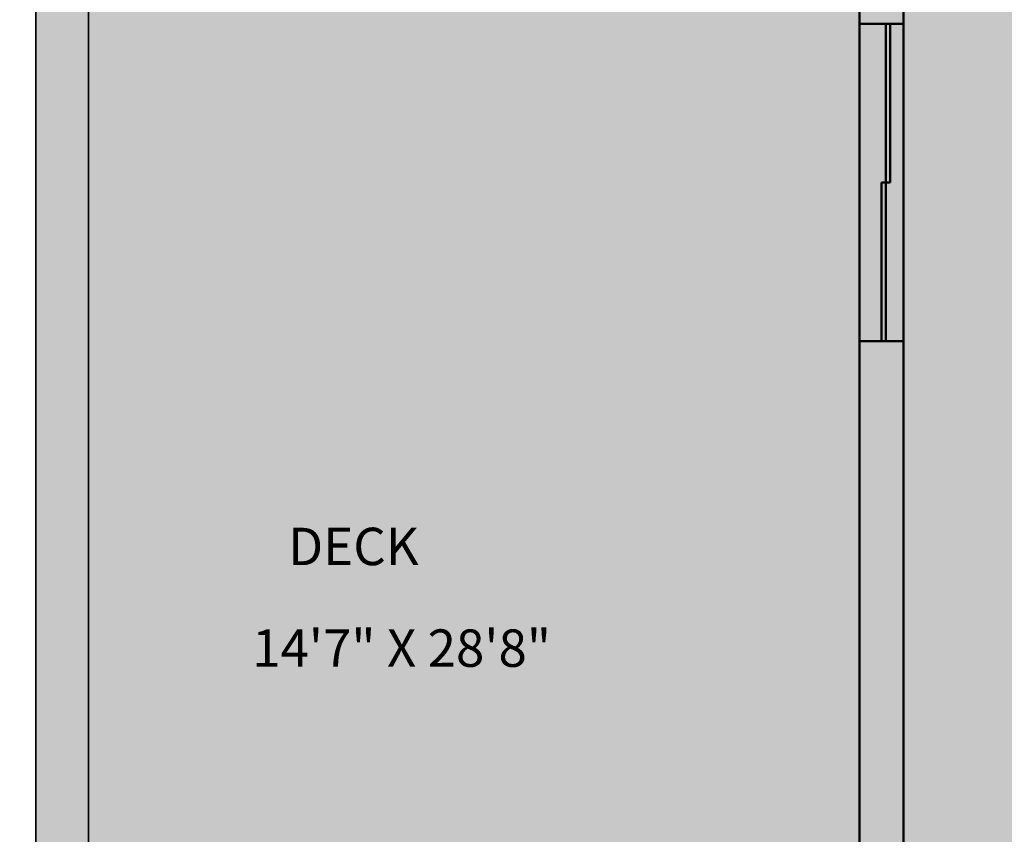
# Model space of a CAD drawing. Units: inches. Extents: x 925 to 2834, y 111 to 1355.
# Tile 14 of 25: x 1069 to 1293, y 882 to 1067. Entities that reach past the tile are written whole.
import ezdxf

# ---------------------------------------------------------------- set-up
doc = ezdxf.new("R2010")
doc.units = ezdxf.units.IN
doc.header["$MEASUREMENT"] = 0
for name, color, linetype, lineweight in [('A-ANNO-DIMS', 2, 'Continuous', 18), ('A-ANNO-TTLB', 7, 'Continuous', 35), ('A-AREA-IDEN', 7, 'Continuous', 18), ('A-FLOR-PATT', 252, 'Continuous', 13), ('A-WALL', 7, 'Continuous', 50), ('A-WALL-PATT', 8, 'Continuous', 13)]:
    doc.layers.add(name, color=color, linetype=linetype, lineweight=lineweight)
doc.styles.get("Standard").update_dxf_attribs({"font": 'arial.ttf'})
doc.dimstyles.get("Standard").update_dxf_attribs({"dimtxt": 6, "dimasz": 3, "dimexe": 0.18, "dimexo": 0.0625, "dimgap": 0.09, "dimtad": 0, "dimtih": 1, "dimtoh": 1, "dimdec": 1, "dimzin": 0, "dimdsep": 46, "dimlunit": 3, "dimtxsty": 'Standard', "dimblk": 'ARCHTICK', "dimcen": 0.09, "dimadec": 0, "dimazin": 0, "dimtfac": 1, "dimtdec": 1, "dimtofl": 0, "dimtmove": 0, "dimatfit": 3, "dimfxl": 1, "dimtolj": 1, "dimtzin": 0, "dimarcsym": 0})

# ---------------------------------------------------------------- blocks, each defined once
blk = doc.blocks.new('_ArchTick')
at = {"color": 0, "linetype": 'ByBlock', "const_width": 0.15}
blk.add_lwpolyline([(-0.5, -0.5), (0.5, 0.5)], dxfattribs=at)
blk = doc.blocks.new('*D36')
at = {"layer": 'A-ANNO-DIMS', "color": 0, "lineweight": -2, "transparency": 16777216}
for p, q in [((1084.65, 1081.59), (934.81, 1081.59)), ((934.99, 1081.59), (934.99, 907.74)), ((934.99, 727.59), (934.99, 901.43)), ((1084.65, 727.59), (934.81, 727.59))]:
    blk.add_line(p, q, dxfattribs=at)
at = {"layer": 'Defpoints', "color": 0, "transparency": 16777216}
for p in [(934.99, 1081.59), (1084.71, 1081.59), (1084.71, 727.59)]:
    blk.add_point(p, dxfattribs=at)
at = {"layer": 'A-ANNO-DIMS', "color": 0, "lineweight": -2, "transparency": 16777216, "xscale": 3, "yscale": 3, "zscale": 3}
for p, rotation in [((934.99, 1081.59), 90), ((934.99, 727.59), 270)]:
    blk.add_blockref('_ArchTick', p, dxfattribs=dict(at, rotation=rotation))
at = {"layer": 'A-ANNO-DIMS', "color": 0, "transparency": 16777216, "insert": (934.99, 904.59), "char_height": 6, "attachment_point": 5}
blk.add_mtext('\\A1;354', dxfattribs=at)

msp = doc.modelspace()

# ---------------------------------------------------------------- hatches: boundary and pattern name
at = {"layer": 'A-FLOR-PATT', "transparency": 33554605}
h = msp.add_hatch(color=256, dxfattribs=at)
h.dxf.hatch_style = 1
h.paths.add_polyline_path([(1931.688, 1294.5638), (991.7375, 1294.5638), (991.7375, 172.1134), (1931.688, 172.1134)])
h.paths.add_polyline_path([(1910.7128, 1273.5886), (1910.7128, 193.0886), (1012.7128, 193.0886), (1012.7128, 1273.5886)], flags=16)
h.paths.add_polyline_path([(1850.7128, 1213.5886), (1850.7128, 253.0886), (1072.7128, 253.0886), (1072.7128, 1213.5886)], flags=0)
h.paths.add_polyline_path([(1838.7128, 1201.5886), (1838.7128, 265.0886), (1084.7128, 265.0886), (1084.7128, 530.5886), (1084.7128, 1201.5886)], flags=0)
h.paths.add_polyline_path([(1547.6758, 1155.7396), (1547.6758, 1119.115), (1513.0687, 1119.115), (1513.0687, 1155.7396)], flags=0)
h.paths.add_polyline_path([(1600.1067, 1154.9439), (1634.7139, 1154.9439), (1634.7139, 1119.115), (1600.1067, 1119.115)], flags=0)
h.paths.add_polyline_path([(1505.2502, 1144.5358), (1505.2502, 1119.115), (1470.643, 1119.115), (1470.643, 1144.5358)], flags=0)
h.paths.add_polyline_path([(1559.1357, 1141.0962), (1593.7428, 1141.0962), (1593.7428, 1119.115), (1559.1357, 1119.115)], flags=0)
h.paths.add_polyline_path([(1462.8966, 1154.9439), (1462.8966, 1119.115), (1428.2895, 1119.115), (1428.2895, 1154.9439)], flags=0)
h.paths.add_polyline_path([(1642.4603, 1144.5358), (1677.0675, 1144.5358), (1677.0675, 1119.115), (1642.4603, 1119.115)], flags=0)
h.paths.add_polyline_path([(1422.3508, 1141.0962), (1422.3508, 1119.115), (1387.7436, 1119.115), (1387.7436, 1141.0962)], flags=0)
h.paths.add_polyline_path([(1684.8859, 1155.7396), (1719.4931, 1155.7396), (1719.4931, 1119.115), (1684.8859, 1119.115)], flags=0)
h.paths.add_polyline_path([(1718.7128, 1081.5886), (1718.7128, 1050.1249), (1715.7128, 1050.1249), (1715.7128, 1026.1249), (1715.7128, 1002.1249), (1718.7128, 1002.1249), (1730.7128, 1002.1249), (1730.7128, 998.1249), (1730.7128, 990.1249), (1730.7128, 986.1249), (1718.7128, 986.1249), (1718.7128, 893.5886), (1715.3735, 893.5886), (1715.3735, 891.5886), (1713.3735, 891.5886, 0.41421356), (1677.3735, 855.5886), (1713.3735, 855.5886), (1713.3735, 853.5886), (1715.3735, 853.5886), (1715.3735, 851.5886), (1718.7128, 851.5886), (1718.7128, 821.5865), (1734.4655, 821.5865), (1734.3735, 819.5886, -0.41421356), (1712.4415, 793.5886), (1712.4415, 791.5886), (1718.7128, 791.5886), (1718.7128, 717.5886), (1718.7128, 669.5886), (1732.7128, 669.5886), (1732.7128, 665.5886), (1732.7128, 641.5886), (1732.7128, 634.5886), (1732.7128, 610.5886), (1732.7128, 603.5886), (1718.7128, 603.5886), (1718.7128, 385.0886), (1434.2128, 385.0886), (1434.2128, 530.5886), (1410.2128, 530.5886), (1408.2128, 530.5886), (1408.2128, 532.5886, 0.41421356), (1372.2128, 568.5886), (1372.2128, 532.5886), (1370.2128, 532.5886), (1370.2128, 530.5886), (1368.2128, 530.5886), (1282.2128, 530.5886), (1210.2128, 530.5886), (1200.2128, 530.5886), (1200.2128, 542.1915), (1183.2307, 542.1915), (1183.2307, 546.1915), (1200.2128, 546.1915), (1200.2128, 572.1915), (1183.2307, 572.1915), (1183.2307, 576.1915), (1200.2128, 576.1915), (1200.2128, 727.5886), (1210.2128, 727.5886), (1234.2128, 727.5886), (1259.7128, 727.5886), (1259.7128, 775.5886), (1259.7128, 799.5886), (1259.7128, 847.5886), (1259.7128, 993.5872), (1259.7128, 1065.5872), (1259.7128, 1071.5886), (1219.6318, 1071.5886), (1219.6318, 1081.5886), (1084.7128, 1081.5886), (1084.7128, 1119.115), (1256.8974, 1119.115), (1256.8974, 1154.9439), (1291.5046, 1154.9439), (1291.5046, 1119.115), (1256.8974, 1119.115), (1256.6723, 1081.5886), (1293.7128, 1081.5886), (1341.7128, 1081.5886), (1341.7128, 1093.5886), (1347.7128, 1093.5886), (1371.7128, 1093.5886), (1377.7128, 1093.5886), (1377.7128, 1081.5886), (1668.7128, 1081.5886), (1668.7128, 1117.5886), (1675.7128, 1117.5886), (1711.7128, 1117.5886), (1718.7128, 1117.5886)], flags=0)
h.paths.add_polyline_path([(1376.2838, 1155.7396), (1376.2838, 1119.115), (1341.6766, 1119.115), (1341.6766, 1155.7396)], flags=0)
h.paths.add_polyline_path([(1341.7128, 1076.0886), (1293.7128, 1076.0886), (1293.7128, 1071.5886), (1269.7128, 1071.5886), (1269.7128, 1065.5872), (1266.7128, 1065.5872), (1266.7128, 1029.5872), (1265.7128, 1029.5872), (1265.7128, 993.5872), (1269.7128, 993.5872), (1269.7128, 903.5886), (1269.7128, 893.5886), (1269.7128, 847.5886), (1265.2128, 847.5886), (1265.2128, 799.5886), (1269.7128, 799.5886), (1269.7128, 775.5886), (1265.2128, 775.5886), (1265.2128, 727.5886), (1269.7128, 727.5886), (1444.2128, 727.5886), (1444.2128, 717.5886), (1234.2128, 717.5886), (1234.2128, 722.0886), (1210.2128, 722.0886), (1210.2128, 717.5886), (1210.2128, 540.5886), (1210.2128, 536.0886), (1282.2128, 536.0886), (1282.2128, 535.0886), (1210.2128, 535.0886), (1210.2128, 540.5886), (1210.2128, 717.5886), (1210.2128, 723.0886), (1234.2128, 723.0886), (1234.2128, 717.5886), (1444.2128, 717.5886), (1444.2128, 727.5886), (1269.7128, 727.5886), (1264.2128, 727.5886), (1264.2128, 775.5886), (1269.7128, 775.5886), (1269.7128, 799.5886), (1264.2128, 799.5886), (1264.2128, 847.5886), (1269.7128, 847.5886), (1269.7128, 893.5886), (1269.7128, 903.5886), (1269.7128, 993.5872), (1264.7128, 993.5872), (1264.7128, 1029.5872), (1265.7128, 1029.5872), (1265.7128, 1065.5872), (1269.7128, 1065.5872), (1269.7128, 1071.5886), (1293.7128, 1071.5886), (1293.7128, 1077.0886), (1341.7128, 1077.0886)], flags=0)
h.paths.add_polyline_path([(1730.9529, 1141.0962), (1765.5601, 1141.0962), (1765.5601, 1119.115), (1730.9529, 1119.115)], flags=0)
h.paths.add_polyline_path([(1333.8582, 1144.5358), (1333.8582, 1119.115), (1299.251, 1119.115), (1299.251, 1144.5358)], flags=0)
h.paths.add_polyline_path([(1592.7128, 968.5886), (1596.0342, 968.5886), (1602.7128, 968.5886), (1708.7128, 968.5886), (1708.7128, 903.5886), (1602.7128, 903.5886), (1602.7128, 938.5886), (1592.7128, 938.5886), (1592.7128, 903.5886), (1451.7128, 903.5886), (1451.7128, 893.5886), (1511.7128, 893.5886), (1511.7128, 881.5886), (1515.2128, 881.5886), (1518.7128, 881.5886), (1518.7128, 893.5886), (1592.7128, 893.5886), (1592.7128, 799.5886), (1518.7128, 799.5886), (1518.7128, 857.5886), (1511.7128, 857.5886), (1511.7128, 799.5886), (1511.7128, 772.0886), (1521.7128, 772.0886), (1521.7128, 792.5886), (1592.7128, 792.5886), (1592.7128, 727.5886), (1521.7128, 727.5886), (1521.7128, 748.0886), (1511.7128, 748.0886), (1511.7128, 717.5886), (1708.7128, 717.5886), (1714.2128, 717.5886), (1714.2128, 669.5886), (1708.7128, 669.5886), (1708.7128, 641.5886), (1492.2128, 641.5886), (1492.2128, 631.5886), (1621.2128, 631.5886), (1621.2128, 443.0886), (1625.7128, 443.0886), (1625.7128, 503.0886), (1625.7128, 507.5886), (1625.7128, 631.5886), (1708.7128, 631.5886), (1708.7128, 507.5886), (1655.7128, 507.5886), (1655.7128, 503.0886), (1708.7128, 503.0886), (1708.7128, 395.0886), (1625.7128, 395.0886), (1625.7128, 419.0886), (1621.2128, 419.0886), (1621.2128, 395.0886), (1482.2128, 395.0886), (1482.2128, 385.0886), (1434.2128, 385.0886), (1434.2128, 433.0886), (1444.2128, 433.0886), (1444.2128, 631.5886), (1450.2128, 631.5886), (1450.2128, 634.91), (1452.2128, 634.91), (1452.2128, 669.5886), (1454.2128, 669.5886, -0.40021217), (1490.1712, 635.3173), (1492.2128, 635.3173), (1492.2128, 641.5886), (1564.7128, 641.5886), (1564.7128, 677.5886), (1672.7128, 677.5886), (1672.7128, 681.5886), (1564.7128, 681.5886), (1564.7128, 717.5886), (1511.7128, 717.5886), (1511.7128, 748.0886), (1511.7128, 772.0886), (1511.7128, 799.5886), (1511.7128, 857.5886), (1511.8913, 857.5886), (1511.8913, 859.5886), (1515.6201, 859.5886, 0.41421356), (1537.552, 879.5886), (1513.552, 879.5886), (1511.8913, 879.5886), (1511.8913, 881.5886), (1511.7128, 881.5886), (1511.7128, 893.5886), (1451.7128, 893.5886), (1451.7128, 903.5886), (1592.7128, 903.5886), (1592.7128, 938.5886), (1592.7128, 940.5886), (1596.4415, 940.5886, 0.41421356), (1618.3735, 966.5886), (1594.3735, 966.5886), (1592.7128, 966.5886)], flags=0)
h.paths.add_polyline_path([(1377.7128, 903.5886), (1377.7128, 893.5886), (1305.7128, 893.5886), (1305.7128, 903.5886)], flags=0)
h.paths.add_polyline_path([(1708.7128, 821.5886), (1712.0342, 821.5886), (1712.0342, 819.5886), (1710.3735, 819.5886), (1708.7128, 819.5886)], flags=0)
h.paths.add_polyline_path([(1576.7128, 695.1992), (1575.5896, 693.6649), (1575.9687, 694.6994), (1575.4438, 695.1992), (1575.9687, 695.699), (1575.5896, 696.7335)], flags=0)
h.paths.add_polyline_path([(1565.9817, 662.3134), (1565.4568, 661.8136), (1565.8359, 660.7791), (1564.7128, 662.3134), (1565.8359, 663.8477), (1565.4568, 662.8132)], flags=0)
h.paths.add_polyline_path([(1444.2128, 433.0886), (1444.2128, 395.0886), (1482.2128, 395.0886), (1482.2128, 389.0886), (1438.2128, 389.0886), (1438.2128, 391.8608), (1438.2128, 433.0886)], flags=0)
h.paths.add_polyline_path([(1410.2128, 506.5886), (1410.2128, 289.0886), (1108.7128, 289.0886), (1108.7128, 506.5886)], flags=0)
h.paths.add_polyline_path([(1612.3153, 838.3016), (1680.4151, 838.3016), (1680.4151, 851.3131), (1612.3153, 851.3131)], flags=8)
h.paths.add_polyline_path([(1208.3174, 395.0436), (1282.1017, 395.0436), (1282.1017, 408.0552), (1208.3174, 408.0552)], flags=8)
h.paths.add_polyline_path([(1291.8049, 598.7427), (1369.8017, 598.7427), (1369.8017, 611.7542), (1291.8049, 611.7542)], flags=8)
h.paths.add_polyline_path([(1119.679, 917.3022), (1191.0817, 917.3022), (1191.0817, 930.3137), (1119.679, 930.3137)], flags=8)
h.paths.add_polyline_path([(1332.2261, 815.9808), (1410.2258, 815.9808), (1410.2258, 829.001), (1332.2261, 829.001)], flags=8)
h.paths.add_polyline_path([(1390.9013, 955.8158), (1475.4981, 955.8158), (1475.4981, 968.8273), (1390.9013, 968.8273)], flags=8)
h.paths.add_polyline_path([(1620.3436, 998.9325), (1688.4434, 998.9325), (1688.4434, 1011.944), (1620.3436, 1011.944)], flags=8)
h.paths.add_polyline_path([(1620.3436, 914.1039), (1691.7405, 914.1039), (1691.7405, 927.1155), (1620.3436, 927.1155)], flags=8)
h.paths.add_polyline_path([(1521.4542, 816.005), (1589.5569, 816.005), (1589.5569, 829.0253), (1521.4542, 829.0253)], flags=8)
h.paths.add_polyline_path([(1528.524, 740.3497), (1602.3082, 740.3497), (1602.3082, 753.3613), (1528.524, 753.3613)], flags=8)
h.paths.add_polyline_path([(1627.6094, 762.6128), (1702.3091, 762.6128), (1702.3091, 775.6244), (1627.6094, 775.6244)], flags=8)
h.paths.add_polyline_path([(1610.5442, 657.2751), (1684.3284, 657.2751), (1684.3284, 670.2867), (1610.5442, 670.2867)], flags=8)
h.paths.add_polyline_path([(1636.6983, 519.472), (1711.3981, 519.472), (1711.3981, 532.4835), (1636.6983, 532.4835)], flags=8)
h.paths.add_polyline_path([(1616.8577, 424.8539), (1694.8545, 424.8539), (1694.8545, 437.8654), (1616.8577, 437.8654)], flags=8)
h.paths.add_polyline_path([(1506.1456, 460.8838), (1579.9299, 460.8838), (1579.9299, 473.8953), (1506.1456, 473.8953)], flags=8)
h.paths.add_polyline_path([(1624.6119, 784.6011), (1696.9185, 784.6011), (1696.9185, 797.7864), (1624.6119, 797.7864)], flags=8)
h.paths.add_polyline_path([(1606.3732, 854.2194), (1683.3039, 854.2194), (1683.3039, 867.4048), (1606.3732, 867.4048)], flags=8)
h.paths.add_polyline_path([(1127.8008, 940.3581), (1165.1637, 940.3581), (1165.1637, 953.5348), (1127.8008, 953.5348)], flags=8)
h.paths.add_polyline_path([(1620.8657, 1019.4968), (1677.3447, 1019.4968), (1677.3447, 1032.6735), (1620.8657, 1032.6735)], flags=8)
h.paths.add_polyline_path([(1620.8643, 930.1821), (1703.0564, 930.1821), (1703.0564, 943.3675), (1620.8643, 943.3675)], flags=8)
h.paths.add_polyline_path([(1324.5702, 836.8338), (1408.0892, 836.8338), (1408.0892, 850.0191), (1324.5702, 850.0191)], flags=8)
h.paths.add_polyline_path([(1281.6584, 622.8885), (1383.6213, 622.8885), (1383.6213, 636.0739), (1281.6584, 636.0739)], flags=8)
h.paths.add_polyline_path([(1210.6721, 416.7893), (1269.1299, 416.7893), (1269.1299, 429.9747), (1210.6721, 429.9747)], flags=8)
h.paths.add_polyline_path([(1507.8264, 477.4836), (1586.7329, 477.4836), (1586.7329, 490.669), (1507.8264, 490.669)], flags=8)
h.paths.add_polyline_path([(1643.6238, 443.8135), (1696.6696, 443.8135), (1696.6696, 456.5643), (1643.6238, 456.5643)], flags=8)
h.paths.add_polyline_path([(1647.2466, 540.5638), (1693.1825, 540.5638), (1693.1825, 553.7491), (1647.2466, 553.7491)], flags=8)
h.paths.add_polyline_path([(1626.0633, 668.5064), (1673.3174, 668.5064), (1673.3174, 681.6831), (1626.0633, 681.6831)], flags=8)
h.paths.add_polyline_path([(1538.2915, 830.7872), (1567.5942, 830.7872), (1567.5942, 843.5293), (1538.2915, 843.5293)], flags=8)
h.paths.add_polyline_path([(1530.9338, 754.0477), (1559.576, 754.0477), (1559.576, 766.7898), (1530.9338, 766.7898)], flags=8)
h.paths.add_polyline_path([(1351.2461, 979.2309), (1513.8919, 979.2309), (1513.8919, 992.4076), (1351.2461, 992.4076)], flags=8)
at = {"layer": 'A-FLOR-PATT'}
h = msp.add_hatch(color=256, dxfattribs=at)
h.dxf.hatch_style = 1
h.paths.add_polyline_path([(1850.7128, 1213.5886), (1072.7128, 1213.5886), (1072.7128, 253.0886), (1850.7128, 253.0886)])
h.paths.add_polyline_path([(1084.7128, 1201.5886), (1838.7128, 1201.5886), (1838.7128, 265.0886), (1084.7128, 265.0886)], flags=16)
h.paths.add_polyline_path([(1183.2307, 576.1915), (1200.2128, 576.1915), (1200.2128, 727.5886), (1210.2128, 727.5886), (1234.2128, 727.5886), (1259.7128, 727.5886), (1259.7128, 775.5886), (1259.7128, 799.5886), (1259.7128, 847.5886), (1259.7128, 993.5872), (1259.7128, 1065.5872), (1259.7128, 1071.5886), (1219.6318, 1071.5886), (1219.6318, 1081.5886), (1293.7128, 1081.5886), (1341.7128, 1081.5886), (1341.7128, 1093.5886), (1347.7128, 1093.5886), (1347.7128, 1081.5886), (1371.7128, 1081.5886), (1371.7128, 1093.5886), (1377.7128, 1093.5886), (1377.7128, 1081.5886), (1668.7128, 1081.5886), (1668.7128, 1117.5886), (1675.7128, 1117.5886), (1675.7128, 1081.5886), (1711.7128, 1081.5886), (1711.7128, 1117.5886), (1718.7128, 1117.5886), (1718.7128, 1081.5886), (1718.7128, 1050.1249), (1715.7128, 1050.1249), (1715.7128, 1026.1249), (1715.7128, 1002.1249), (1718.7128, 1002.1249), (1730.7128, 1002.1249), (1730.7128, 998.1249), (1730.7128, 990.1249), (1730.7128, 986.1249), (1718.7128, 986.1249), (1718.7128, 893.5886), (1715.3735, 893.5886), (1715.3735, 891.5886), (1713.3735, 891.5886, 0.41421356), (1677.3735, 855.5886), (1713.3735, 855.5886), (1713.3735, 853.5886), (1715.3735, 853.5886), (1715.3735, 851.5886), (1718.7128, 851.5886), (1718.7128, 821.5865), (1734.4655, 821.5865), (1734.3735, 819.5886, -0.41421356), (1712.4415, 793.5886), (1712.4415, 791.5886), (1718.7128, 791.5886), (1718.7128, 717.5886), (1718.7128, 669.5886), (1732.7128, 669.5886), (1732.7128, 665.5886), (1732.7128, 641.5886), (1732.7128, 634.5886), (1732.7128, 610.5886), (1732.7128, 603.5886), (1718.7128, 603.5886), (1718.7128, 385.0886), (1434.2128, 385.0886), (1434.2128, 433.0886), (1434.2128, 530.5886), (1410.2128, 530.5886), (1408.2128, 530.5886), (1408.2128, 532.5886, 0.41421356), (1372.2128, 568.5886), (1372.2128, 532.5886), (1370.2128, 532.5886), (1370.2128, 530.5886), (1368.2128, 530.5886), (1282.2128, 530.5886), (1210.2128, 530.5886), (1200.2128, 530.5886), (1200.2128, 542.1915), (1183.2307, 542.1915), (1183.2307, 546.1915), (1200.2128, 546.1915), (1200.2128, 572.1915), (1183.2307, 572.1915)], flags=0)
h.paths.add_polyline_path([(1210.2128, 717.5886), (1210.2128, 723.0886), (1234.2128, 723.0886), (1234.2128, 717.5886), (1444.2128, 717.5886), (1444.2128, 727.5886), (1269.7128, 727.5886), (1264.2128, 727.5886), (1264.2128, 775.5886), (1269.7128, 775.5886), (1269.7128, 799.5886), (1264.2128, 799.5886), (1264.2128, 847.5886), (1269.7128, 847.5886), (1269.7128, 893.5886), (1269.7128, 903.5886), (1269.7128, 993.5872), (1264.7128, 993.5872), (1264.7128, 1029.5872), (1265.7128, 1029.5872), (1265.7128, 1065.5872), (1269.7128, 1065.5872), (1269.7128, 1071.5886), (1293.7128, 1071.5886), (1293.7128, 1077.0886), (1341.7128, 1077.0886), (1341.7128, 1076.0886), (1293.7128, 1076.0886), (1293.7128, 1071.5886), (1269.7128, 1071.5886), (1269.7128, 1065.5872), (1266.7128, 1065.5872), (1266.7128, 1029.5872), (1265.7128, 1029.5872), (1265.7128, 993.5872), (1269.7128, 993.5872), (1269.7128, 903.5886), (1269.7128, 893.5886), (1269.7128, 847.5886), (1265.2128, 847.5886), (1265.2128, 799.5886), (1269.7128, 799.5886), (1269.7128, 775.5886), (1265.2128, 775.5886), (1265.2128, 727.5886), (1269.7128, 727.5886), (1444.2128, 727.5886), (1444.2128, 717.5886), (1234.2128, 717.5886), (1234.2128, 722.0886), (1210.2128, 722.0886), (1210.2128, 717.5886), (1210.2128, 540.5886), (1210.2128, 536.0886), (1282.2128, 536.0886), (1282.2128, 535.0886), (1210.2128, 535.0886), (1210.2128, 540.5886)], flags=0)
h.paths.add_polyline_path([(1450.2128, 634.91), (1452.2128, 634.91), (1452.2128, 669.5886), (1454.2128, 669.5886, -0.40021217), (1490.1712, 635.3173), (1492.2128, 635.3173), (1492.2128, 641.5886), (1564.7128, 641.5886), (1564.7128, 677.5886), (1672.7128, 677.5886), (1672.7128, 681.5886), (1564.7128, 681.5886), (1564.7128, 717.5886), (1511.7128, 717.5886), (1511.7128, 748.0886), (1511.7128, 772.0886), (1511.7128, 799.5886), (1511.7128, 857.5886), (1511.8913, 857.5886), (1511.8913, 859.5886), (1515.6201, 859.5886, 0.41421356), (1537.552, 879.5886), (1513.552, 879.5886), (1511.8913, 879.5886), (1511.8913, 881.5886), (1511.7128, 881.5886), (1511.7128, 893.5886), (1451.7128, 893.5886), (1451.7128, 903.5886), (1592.7128, 903.5886), (1592.7128, 938.5886), (1592.7128, 940.5886), (1596.4415, 940.5886, 0.41421356), (1618.3735, 966.5886), (1594.3735, 966.5886), (1592.7128, 966.5886), (1592.7128, 968.5886), (1596.0342, 968.5886), (1602.7128, 968.5886), (1708.7128, 968.5886), (1708.7128, 903.5886), (1602.7128, 903.5886), (1602.7128, 938.5886), (1592.7128, 938.5886), (1592.7128, 903.5886), (1451.7128, 903.5886), (1451.7128, 893.5886), (1511.7128, 893.5886), (1511.7128, 881.5886), (1518.7128, 881.5886), (1518.7128, 893.5886), (1592.7128, 893.5886), (1592.7128, 799.5886), (1518.7128, 799.5886), (1518.7128, 857.5886), (1511.7128, 857.5886), (1511.7128, 799.5886), (1511.7128, 772.0886), (1521.7128, 772.0886), (1521.7128, 792.5886), (1592.7128, 792.5886), (1592.7128, 727.5886), (1521.7128, 727.5886), (1521.7128, 748.0886), (1511.7128, 748.0886), (1511.7128, 717.5886), (1708.7128, 717.5886), (1714.2128, 717.5886), (1714.2128, 669.5886), (1708.7128, 669.5886), (1708.7128, 641.5886), (1492.2128, 641.5886), (1492.2128, 631.5886), (1621.2128, 631.5886), (1621.2128, 443.0886), (1625.7128, 443.0886), (1625.7128, 503.0886), (1625.7128, 507.5886), (1625.7128, 631.5886), (1708.7128, 631.5886), (1708.7128, 507.5886), (1655.7128, 507.5886), (1655.7128, 503.0886), (1708.7128, 503.0886), (1708.7128, 395.0886), (1625.7128, 395.0886), (1625.7128, 419.0886), (1621.2128, 419.0886), (1621.2128, 395.0886), (1482.2128, 395.0886), (1482.2128, 389.0886), (1438.2128, 389.0886), (1438.2128, 391.8608), (1438.2128, 433.0886), (1444.2128, 433.0886), (1444.2128, 631.5886), (1450.2128, 631.5886)], flags=0)
h.paths.add_polyline_path([(1444.2128, 433.0886), (1444.2128, 395.0886), (1482.2128, 395.0886), (1482.2128, 391.0886), (1440.2128, 391.0886), (1440.2128, 391.8608), (1440.2128, 433.0886)], flags=0)
h.paths.add_polyline_path([(1305.7128, 893.5886), (1305.7128, 903.5886), (1377.7128, 903.5886), (1377.7128, 893.5886)], flags=0)
h.paths.add_polyline_path([(1564.7128, 662.3134), (1565.8359, 663.8477), (1565.4568, 662.8132), (1565.9817, 662.3134), (1565.4568, 661.8136), (1565.8359, 660.7791)], flags=0)
h.paths.add_polyline_path([(1575.4438, 695.1992), (1575.9687, 695.699), (1575.5896, 696.7335), (1576.7128, 695.1992), (1575.5896, 693.6649), (1575.9687, 694.6994)], flags=0)
h.paths.add_polyline_path([(1708.7128, 821.5886), (1712.0342, 821.5886), (1712.0342, 819.5886), (1710.3735, 819.5886), (1708.7128, 819.5886)], flags=0)
h = msp.add_hatch(color=256, dxfattribs=at)
h.dxf.hatch_style = 1
h.paths.add_polyline_path([(1718.7128, 603.5886), (1708.7128, 603.5886), (1708.7128, 507.5886), (1655.7128, 507.5886), (1655.7128, 503.0886), (1708.7128, 503.0886), (1708.7128, 395.0886), (1625.7128, 395.0886), (1625.7128, 419.0886), (1621.2128, 419.0886), (1621.2128, 395.0886), (1482.2128, 395.0886), (1482.2128, 385.0886), (1718.7128, 385.0886)])
h.paths.add_polyline_path([(1625.7128, 631.5886), (1708.7128, 631.5886), (1708.7128, 603.5886), (1718.7128, 603.5886), (1732.7128, 603.5886), (1732.7128, 610.5886), (1715.7128, 610.5886), (1715.7128, 634.5886), (1732.7128, 634.5886), (1732.7128, 641.5886), (1715.7128, 641.5886), (1715.7128, 665.5886), (1732.7128, 665.5886), (1732.7128, 669.5886), (1708.7128, 669.5886), (1708.7128, 641.5886), (1492.2128, 641.5886), (1492.2128, 631.5886), (1621.2128, 631.5886), (1621.2128, 443.0886), (1625.7128, 443.0886), (1625.7128, 503.0886), (1625.7128, 507.5886)])
h.paths.add_polyline_path([(1718.7128, 851.5886), (1708.7128, 851.5886), (1708.7128, 828.5886), (1602.7128, 828.5886), (1602.7128, 893.5886), (1708.7128, 893.5886), (1718.7128, 893.5886), (1718.7128, 986.1249), (1730.7128, 986.1249), (1730.7128, 990.1249), (1718.7128, 990.1249), (1718.7128, 998.1249), (1730.7128, 998.1249), (1730.7128, 1002.1249), (1718.7128, 1002.1249), (1708.7128, 1002.1249), (1708.7128, 975.5886), (1602.7128, 975.5886), (1602.7128, 1011.5886), (1592.7128, 1011.5886), (1592.7128, 968.5886), (1596.0342, 968.5886), (1602.7128, 968.5886), (1708.7128, 968.5886), (1708.7128, 903.5886), (1602.7128, 903.5886), (1602.7128, 938.5886), (1592.7128, 938.5886), (1592.7128, 903.5886), (1451.7128, 903.5886), (1451.7128, 893.5886), (1511.7128, 893.5886), (1511.7128, 881.5886), (1515.2128, 881.5886), (1518.7128, 881.5886), (1518.7128, 893.5886), (1592.7128, 893.5886), (1592.7128, 799.5886), (1518.7128, 799.5886), (1518.7128, 857.5886), (1511.7128, 857.5886), (1511.7128, 799.5886), (1511.7128, 772.0886), (1521.7128, 772.0886), (1521.7128, 792.5886), (1592.7128, 792.5886), (1592.7128, 727.5886), (1521.7128, 727.5886), (1521.7128, 748.0886), (1511.7128, 748.0886), (1511.7128, 717.5886), (1708.7128, 717.5886), (1718.7128, 717.5886), (1718.7128, 727.5886), (1718.7128, 791.5886), (1708.7128, 791.5886), (1708.7128, 727.5886), (1602.7128, 727.5886), (1602.7128, 821.5886), (1708.7128, 821.5886), (1712.0342, 821.5886), (1718.7128, 821.5886)])
h.paths.add_polyline_path([(1718.7128, 1081.5886), (1718.7128, 1117.5886), (1711.7128, 1117.5886), (1711.7128, 1081.5886), (1675.7128, 1081.5886), (1675.7128, 1117.5886), (1668.7128, 1117.5886), (1668.7128, 1081.5886), (1377.7128, 1081.5886), (1377.7128, 1093.5886), (1371.7128, 1093.5886), (1371.7128, 1081.5886), (1347.7128, 1081.5886), (1347.7128, 1093.5886), (1341.7128, 1093.5886), (1341.7128, 1081.5886), (1341.7128, 1071.5886), (1592.7128, 1071.5886), (1592.7128, 1035.5886), (1602.7128, 1035.5886), (1602.7128, 1071.5886), (1708.7128, 1071.5886), (1708.7128, 1050.1249), (1718.7128, 1050.1249)])
h.paths.add_polyline_path([(1293.7128, 1081.5886), (1219.6318, 1081.5886), (1219.6318, 1071.5886), (1259.7128, 1071.5886), (1259.7128, 1065.5872), (1269.7128, 1065.5872), (1269.7128, 1071.5886), (1293.7128, 1071.5886)])
h.paths.add_polyline_path([(1269.7128, 903.5886), (1269.7128, 993.5872), (1259.7128, 993.5872), (1259.7128, 847.5886), (1269.7128, 847.5886), (1269.7128, 893.5886)])
h.paths.add_polyline_path([(1377.7128, 903.5886), (1305.7128, 903.5886), (1305.7128, 893.5886), (1377.7128, 893.5886)])
h.paths.add_polyline_path([(1444.2128, 727.5886), (1269.7128, 727.5886), (1259.7128, 727.5886), (1234.2128, 727.5886), (1234.2128, 717.5886), (1444.2128, 717.5886)])
h.paths.add_polyline_path([(1269.7128, 799.5886), (1259.7128, 799.5886), (1259.7128, 775.5886), (1269.7128, 775.5886)])
h.paths.add_polyline_path([(1444.2128, 631.5886), (1450.2128, 631.5886), (1450.2128, 634.91), (1450.2128, 641.5886), (1434.2128, 641.5886), (1434.2128, 540.5886), (1410.2128, 540.5886), (1410.2128, 530.5886), (1434.2128, 530.5886), (1434.2128, 433.0886), (1444.2128, 433.0886)])
h.paths.add_polyline_path([(1368.2128, 533.91), (1368.2128, 540.5886), (1282.2128, 540.5886), (1282.2128, 530.5886), (1368.2128, 530.5886)])
h.paths.add_polyline_path([(1210.2128, 717.5886), (1210.2128, 727.5886), (1200.2128, 727.5886), (1200.2128, 576.1915), (1183.2307, 576.1915), (1183.2307, 572.1915), (1200.2128, 572.1915), (1200.2128, 546.1915), (1183.2307, 546.1915), (1183.2307, 542.1915), (1200.2128, 542.1915), (1200.2128, 530.5886), (1210.2128, 530.5886), (1210.2128, 540.5886)])
at = {"layer": 'A-FLOR-PATT', "transparency": 33554574}
h = msp.add_hatch(color=256, dxfattribs=at)
h.dxf.hatch_style = 1
h.paths.add_polyline_path([(1259.7128, 993.5872), (1259.7128, 1065.5872), (1259.7128, 1071.5886), (1219.6318, 1071.5886), (1219.6318, 1081.5886), (1084.7128, 1081.5886), (1084.7128, 727.5886), (1200.2128, 727.5886), (1210.2128, 727.5886), (1234.2128, 727.5886), (1259.7128, 727.5886), (1259.7128, 775.5886), (1259.7128, 799.5886), (1259.7128, 847.5886)])
at = {"layer": 'A-FLOR-PATT', "transparency": 33554605}
h = msp.add_hatch(color=256, dxfattribs=at)
h.dxf.hatch_style = 1
h.paths.add_polyline_path([(1592.7128, 938.5886), (1592.7128, 940.5886), (1596.4415, 940.5886, 0.41421356), (1618.3735, 966.5886), (1594.3735, 966.5886), (1592.7128, 966.5886), (1592.7128, 968.5886), (1592.7128, 1011.5886), (1602.7128, 1011.5886), (1602.7128, 975.5886), (1708.7128, 975.5886), (1708.7128, 1002.1249), (1711.7128, 1002.1249), (1711.7128, 1026.1249), (1711.7128, 1050.1249), (1708.7128, 1050.1249), (1708.7128, 1071.5886), (1602.7128, 1071.5886), (1602.7128, 1035.5886), (1592.7128, 1035.5886), (1592.7128, 1071.5886), (1341.7128, 1071.5886), (1293.7128, 1071.5886), (1269.7128, 1071.5886), (1269.7128, 1065.5872), (1269.7128, 993.5872), (1269.7128, 903.5886), (1269.7128, 893.5886), (1269.7128, 847.5886), (1269.7128, 799.5886), (1269.7128, 775.5886), (1269.7128, 727.5886), (1444.2128, 727.5886), (1444.2128, 717.5886), (1234.2128, 717.5886), (1210.2128, 717.5886), (1210.2128, 540.5886), (1282.2128, 540.5886), (1368.2128, 540.5886), (1368.2128, 533.91), (1370.2128, 533.91), (1370.2128, 568.5886), (1372.2128, 568.5886, -0.40021217), (1408.1712, 534.3173), (1410.2128, 534.3173), (1410.2128, 540.5886), (1434.2128, 540.5886), (1434.2128, 641.5886), (1450.2128, 641.5886), (1450.2128, 634.91), (1452.2128, 634.91), (1452.2128, 669.5886), (1454.2128, 669.5886, -0.40021217), (1490.1712, 635.3173), (1492.2128, 635.3173), (1492.2128, 641.5886), (1564.7128, 641.5886), (1564.7128, 677.5886), (1672.7128, 677.5886), (1672.7128, 681.5886), (1564.7128, 681.5886), (1564.7128, 717.5886), (1511.7128, 717.5886), (1511.7128, 748.0886), (1511.7128, 772.0886), (1511.7128, 799.5886), (1511.7128, 857.5886), (1511.8913, 857.5886), (1511.8913, 859.5886), (1515.6201, 859.5886, 0.41421356), (1537.552, 879.5886), (1513.552, 879.5886), (1511.8913, 879.5886), (1511.8913, 881.5886), (1511.7128, 881.5886), (1511.7128, 893.5886), (1451.7128, 893.5886), (1451.7128, 903.5886), (1592.7128, 903.5886)])
h.paths.add_polyline_path([(1377.7128, 903.5886), (1377.7128, 893.5886), (1305.7128, 893.5886), (1305.7128, 903.5886)], flags=16)
h.paths.add_polyline_path([(1592.7128, 893.5886), (1518.7128, 893.5886), (1518.7128, 881.5865), (1537.6441, 881.5865), (1537.552, 879.5886, -0.41421356), (1515.6201, 859.5886), (1515.6201, 857.5886), (1518.7128, 857.5886), (1518.7128, 799.5886), (1592.7128, 799.5886)], flags=17)
h.paths.add_polyline_path([(1291.8049, 598.7427), (1369.8017, 598.7427), (1369.8017, 611.7542), (1291.8049, 611.7542)], flags=24)
h.paths.add_polyline_path([(1332.2261, 815.9808), (1410.2258, 815.9808), (1410.2258, 829.001), (1332.2261, 829.001)], flags=24)
h.paths.add_polyline_path([(1390.9013, 955.8158), (1475.4981, 955.8158), (1475.4981, 968.8273), (1390.9013, 968.8273)], flags=24)
h.paths.add_polyline_path([(1620.3436, 998.9325), (1688.4434, 998.9325), (1688.4434, 1011.944), (1620.3436, 1011.944)], flags=24)
h.paths.add_polyline_path([(1620.8657, 1019.4968), (1677.3447, 1019.4968), (1677.3447, 1032.6735), (1620.8657, 1032.6735)], flags=24)
h.paths.add_polyline_path([(1324.5702, 836.8338), (1408.0892, 836.8338), (1408.0892, 850.0191), (1324.5702, 850.0191)], flags=24)
h.paths.add_polyline_path([(1281.6584, 622.8885), (1383.6213, 622.8885), (1383.6213, 636.0739), (1281.6584, 636.0739)], flags=24)
h.paths.add_polyline_path([(1626.0633, 668.5064), (1673.3174, 668.5064), (1673.3174, 681.6831), (1626.0633, 681.6831)], flags=25)
h.paths.add_polyline_path([(1351.2461, 979.2309), (1513.8919, 979.2309), (1513.8919, 992.4076), (1351.2461, 992.4076)], flags=24)
h.paths.add_polyline_path([(1521.4542, 816.005), (1589.5569, 816.005), (1589.5569, 829.0253), (1521.4542, 829.0253)], flags=24)
h.paths.add_polyline_path([(1538.2915, 830.7872), (1567.5942, 830.7872), (1567.5942, 843.5293), (1538.2915, 843.5293)], flags=24)
h.paths.add_polyline_path([(1636.6983, 519.472), (1711.3981, 519.472), (1711.3981, 532.4835), (1636.6983, 532.4835)], flags=9)
h.paths.add_polyline_path([(1616.8577, 424.8539), (1694.8545, 424.8539), (1694.8545, 437.8654), (1616.8577, 437.8654)], flags=9)
h.paths.add_polyline_path([(1506.1456, 460.8838), (1579.9299, 460.8838), (1579.9299, 473.8953), (1506.1456, 473.8953)], flags=9)
h.paths.add_polyline_path([(1606.3732, 854.2194), (1683.3039, 854.2194), (1683.3039, 867.4048), (1606.3732, 867.4048)], flags=25)
h.paths.add_polyline_path([(1507.8264, 477.4836), (1586.7329, 477.4836), (1586.7329, 490.669), (1507.8264, 490.669)], flags=9)
h.paths.add_polyline_path([(1643.6238, 443.8135), (1696.6696, 443.8135), (1696.6696, 456.5643), (1643.6238, 456.5643)], flags=9)
h.paths.add_polyline_path([(1647.2466, 540.5638), (1693.1825, 540.5638), (1693.1825, 553.7491), (1647.2466, 553.7491)], flags=25)
h = msp.add_hatch(color=256, dxfattribs=at)
h.dxf.hatch_style = 1
h.paths.add_polyline_path([(1200.2128, 727.5886), (1084.7128, 727.5886), (1084.7128, 530.5886), (1200.2128, 530.5886), (1200.2128, 542.1915), (1183.2307, 542.1915), (1183.2307, 546.1915), (1200.2128, 546.1915), (1200.2128, 572.1915), (1183.2307, 572.1915), (1183.2307, 576.1915), (1200.2128, 576.1915)])
h.paths.add_polyline_path([(1612.3153, 838.3016), (1680.4151, 838.3016), (1680.4151, 851.3131), (1612.3153, 851.3131)], flags=9)
h.paths.add_polyline_path([(1291.8049, 598.7427), (1369.8017, 598.7427), (1369.8017, 611.7542), (1291.8049, 611.7542)], flags=9)
h.paths.add_polyline_path([(1119.679, 917.3022), (1191.0817, 917.3022), (1191.0817, 930.3137), (1119.679, 930.3137)], flags=9)
h.paths.add_polyline_path([(1332.2261, 815.9808), (1410.2258, 815.9808), (1410.2258, 829.001), (1332.2261, 829.001)], flags=9)
h.paths.add_polyline_path([(1390.9013, 955.8158), (1475.4981, 955.8158), (1475.4981, 968.8273), (1390.9013, 968.8273)], flags=9)
h.paths.add_polyline_path([(1620.3436, 998.9325), (1688.4434, 998.9325), (1688.4434, 1011.944), (1620.3436, 1011.944)], flags=9)
h.paths.add_polyline_path([(1620.3436, 914.1039), (1691.7405, 914.1039), (1691.7405, 927.1155), (1620.3436, 927.1155)], flags=9)
h.paths.add_polyline_path([(1521.4542, 816.005), (1589.5569, 816.005), (1589.5569, 829.0253), (1521.4542, 829.0253)], flags=9)
h.paths.add_polyline_path([(1522.4337, 740.3497), (1596.218, 740.3497), (1596.218, 753.3613), (1522.4337, 753.3613)], flags=9)
h.paths.add_polyline_path([(1606.3732, 854.2194), (1683.3039, 854.2194), (1683.3039, 867.4048), (1606.3732, 867.4048)], flags=9)
h.paths.add_polyline_path([(1127.8008, 940.3581), (1165.1637, 940.3581), (1165.1637, 953.5348), (1127.8008, 953.5348)], flags=9)
h.paths.add_polyline_path([(1620.8657, 1019.4968), (1677.3447, 1019.4968), (1677.3447, 1032.6735), (1620.8657, 1032.6735)], flags=9)
h.paths.add_polyline_path([(1620.8643, 930.1821), (1703.0564, 930.1821), (1703.0564, 943.3675), (1620.8643, 943.3675)], flags=9)
h.paths.add_polyline_path([(1324.5702, 836.8338), (1408.0892, 836.8338), (1408.0892, 850.0191), (1324.5702, 850.0191)], flags=9)
h.paths.add_polyline_path([(1281.6584, 622.8885), (1383.6213, 622.8885), (1383.6213, 636.0739), (1281.6584, 636.0739)], flags=9)
h.paths.add_polyline_path([(1626.0633, 668.5064), (1673.3174, 668.5064), (1673.3174, 681.6831), (1626.0633, 681.6831)], flags=9)
h.paths.add_polyline_path([(1538.2915, 830.7872), (1567.5942, 830.7872), (1567.5942, 843.5293), (1538.2915, 843.5293)], flags=9)
h.paths.add_polyline_path([(1351.2461, 979.2309), (1513.8919, 979.2309), (1513.8919, 992.4076), (1351.2461, 992.4076)], flags=9)
h = msp.add_hatch(color=256, dxfattribs=at)
h.dxf.hatch_style = 1
h.paths.add_polyline_path([(1621.2128, 631.5886), (1492.2128, 631.5886), (1490.2128, 631.5886), (1490.2128, 633.5886, 0.41421356), (1454.2128, 669.5886), (1454.2128, 633.5886), (1452.2128, 633.5886), (1452.2128, 631.5886), (1450.2128, 631.5886), (1444.2128, 631.5886), (1444.2128, 395.0886), (1482.2128, 395.0886), (1621.2128, 395.0886), (1621.2128, 419.0886), (1625.7128, 419.0886), (1625.7128, 395.0886), (1708.7128, 395.0886), (1708.7128, 503.0886), (1655.7128, 503.0886), (1655.7128, 507.5886), (1708.7128, 507.5886), (1708.7128, 631.5886), (1625.7128, 631.5886), (1625.7128, 507.5886), (1625.7128, 503.0886), (1625.7128, 443.0886), (1621.2128, 443.0886)])
h.paths.add_polyline_path([(1636.6983, 519.472), (1711.3981, 519.472), (1711.3981, 532.4835), (1636.6983, 532.4835)], flags=9)
h.paths.add_polyline_path([(1616.8577, 424.8539), (1694.8545, 424.8539), (1694.8545, 437.8654), (1616.8577, 437.8654)], flags=24)
h.paths.add_polyline_path([(1506.1456, 460.8838), (1579.9299, 460.8838), (1579.9299, 473.8953), (1506.1456, 473.8953)], flags=24)
h.paths.add_polyline_path([(1507.8264, 477.4836), (1586.7329, 477.4836), (1586.7329, 490.669), (1507.8264, 490.669)], flags=24)
h.paths.add_polyline_path([(1643.6238, 443.8135), (1696.6696, 443.8135), (1696.6696, 456.5643), (1643.6238, 456.5643)], flags=24)
h.paths.add_polyline_path([(1647.2466, 540.5638), (1693.1825, 540.5638), (1693.1825, 553.7491), (1647.2466, 553.7491)], flags=24)
h.paths.add_polyline_path([(1612.3153, 838.3016), (1680.4151, 838.3016), (1680.4151, 851.3131), (1612.3153, 851.3131)], flags=9)
h.paths.add_polyline_path([(1291.8049, 598.7427), (1369.8017, 598.7427), (1369.8017, 611.7542), (1291.8049, 611.7542)], flags=9)
h.paths.add_polyline_path([(1119.679, 917.3022), (1191.0817, 917.3022), (1191.0817, 930.3137), (1119.679, 930.3137)], flags=9)
h.paths.add_polyline_path([(1332.2261, 815.9808), (1410.2258, 815.9808), (1410.2258, 829.001), (1332.2261, 829.001)], flags=9)
h.paths.add_polyline_path([(1390.9013, 955.8158), (1475.4981, 955.8158), (1475.4981, 968.8273), (1390.9013, 968.8273)], flags=9)
h.paths.add_polyline_path([(1620.3436, 998.9325), (1688.4434, 998.9325), (1688.4434, 1011.944), (1620.3436, 1011.944)], flags=9)
h.paths.add_polyline_path([(1620.3436, 914.1039), (1691.7405, 914.1039), (1691.7405, 927.1155), (1620.3436, 927.1155)], flags=9)
h.paths.add_polyline_path([(1521.4542, 816.005), (1589.5569, 816.005), (1589.5569, 829.0253), (1521.4542, 829.0253)], flags=9)
h.paths.add_polyline_path([(1528.524, 740.3497), (1602.3082, 740.3497), (1602.3082, 753.3613), (1528.524, 753.3613)], flags=9)
h.paths.add_polyline_path([(1627.6094, 762.6128), (1702.3091, 762.6128), (1702.3091, 775.6244), (1627.6094, 775.6244)], flags=9)
h.paths.add_polyline_path([(1624.6119, 784.6011), (1696.9185, 784.6011), (1696.9185, 797.7864), (1624.6119, 797.7864)], flags=9)
h.paths.add_polyline_path([(1606.3732, 854.2194), (1683.3039, 854.2194), (1683.3039, 867.4048), (1606.3732, 867.4048)], flags=9)
h.paths.add_polyline_path([(1127.8008, 940.3581), (1165.1637, 940.3581), (1165.1637, 953.5348), (1127.8008, 953.5348)], flags=9)
h.paths.add_polyline_path([(1620.8657, 1019.4968), (1677.3447, 1019.4968), (1677.3447, 1032.6735), (1620.8657, 1032.6735)], flags=9)
h.paths.add_polyline_path([(1620.8643, 930.1821), (1703.0564, 930.1821), (1703.0564, 943.3675), (1620.8643, 943.3675)], flags=9)
h.paths.add_polyline_path([(1324.5702, 836.8338), (1408.0892, 836.8338), (1408.0892, 850.0191), (1324.5702, 850.0191)], flags=9)
h.paths.add_polyline_path([(1281.6584, 622.8885), (1383.6213, 622.8885), (1383.6213, 636.0739), (1281.6584, 636.0739)], flags=9)
h.paths.add_polyline_path([(1626.0633, 668.5064), (1673.3174, 668.5064), (1673.3174, 681.6831), (1626.0633, 681.6831)], flags=9)
h.paths.add_polyline_path([(1538.2915, 830.7872), (1567.5942, 830.7872), (1567.5942, 843.5293), (1538.2915, 843.5293)], flags=9)
h.paths.add_polyline_path([(1530.9338, 754.0477), (1559.576, 754.0477), (1559.576, 766.7898), (1530.9338, 766.7898)], flags=9)
h.paths.add_polyline_path([(1351.2461, 979.2309), (1513.8919, 979.2309), (1513.8919, 992.4076), (1351.2461, 992.4076)], flags=9)
at = {"layer": 'A-WALL-PATT'}
h = msp.add_hatch(color=256, dxfattribs=at)
h.dxf.hatch_style = 1
h.paths.add_polyline_path([(1259.7128, 1065.5872), (1259.7128, 993.5872), (1264.7128, 993.5872), (1264.7128, 1029.5872), (1265.7128, 1029.5872), (1265.7128, 1065.5872)])
h.paths.add_polyline_path([(1265.7128, 1029.5872), (1265.7128, 993.5872), (1269.7128, 993.5872), (1269.7128, 1065.5872), (1266.7128, 1065.5872), (1266.7128, 1029.5872)])
h = msp.add_hatch(color=256, dxfattribs=at)
h.dxf.hatch_style = 1
h.paths.add_polyline_path([(1264.7128, 1029.5872), (1264.7128, 993.5872), (1265.7128, 993.5872), (1265.7128, 1029.5872)])
h.paths.add_polyline_path([(1265.7128, 1065.5872), (1265.7128, 1029.5872), (1266.7128, 1029.5872), (1266.7128, 1065.5872)])

# ---------------------------------------------------------------- linework, layer by layer
at = {"layer": 'A-ANNO-TTLB'}
for points in [[(1072.7128, 253.0886), (1850.7128, 253.0886), (1850.7128, 1213.5886), (1072.7128, 1213.5886)], [(1084.7128, 265.0886), (1838.7128, 265.0886), (1838.7128, 1201.5886), (1084.7128, 1201.5886)]]:
    msp.add_lwpolyline(points, close=True, dxfattribs=at)
at = {"layer": 'A-WALL'}
for p, q in [((1259.7128, 1071.5886), (1259.7128, 1065.5872)), ((1269.7128, 1071.5886), (1269.7128, 1065.5872)), ((1259.7128, 1065.5872), (1269.7128, 1065.5872)), ((1265.7128, 1065.5872), (1265.7128, 1029.5872)), ((1266.7128, 1029.5872), (1266.7128, 1065.5872)), ((1264.7128, 993.5872), (1264.7128, 1029.5872)), ((1264.7128, 1029.5872), (1265.7128, 1029.5872)), ((1264.7128, 1029.5872), (1265.7128, 1029.5872)), ((1265.7128, 1029.5872), (1265.7128, 993.5872)), ((1265.7128, 1029.5872), (1266.7128, 1029.5872)), ((1265.7128, 1029.5872), (1266.7128, 1029.5872)), ((1259.7128, 993.5872), (1269.7128, 993.5872)), ((1259.7128, 993.5872), (1259.7128, 847.5886)), ((1269.7128, 993.5872), (1269.7128, 903.5886)), ((1269.7128, 893.5886), (1269.7128, 903.5886)), ((1269.7128, 893.5886), (1269.7128, 847.5886))]:
    msp.add_line(p, q, dxfattribs=at)
msp.add_lwpolyline([(1269.7128, 993.5872), (1269.7128, 1065.5872), (1259.7128, 1065.5872), (1259.7128, 993.5872)], close=True, dxfattribs=at)

# ---------------------------------------------------------------- texts
at = {"layer": 'A-AREA-IDEN'}
for s, height, p in [('DECK', 8.49473, (1129.9969, 942.6991)), ('14\'7" X 28\'8"', 8.494735, (1121.8476, 919.6157))]:
    msp.add_text(s, height=height, dxfattribs=at).set_placement(p)

# ---------------------------------------------------------------- dimensions: what is measured, and where the dimension line sits
at = {"layer": 'A-ANNO-DIMS'}
dim = msp.add_linear_dim(base=(934.9875, 1081.5886), p1=(1084.7128, 727.5886), p2=(1084.7128, 1081.5886), angle=90, dimstyle='Standard', override={"dimdec": 0, "dimlfac": 1, "dimrnd": 0, "dimzin": 0, "dimdsep": 46, "dimlunit": 2}, dxfattribs=at)
dim.commit()
dim.dimension.update_dxf_attribs({"geometry": '*D36', "text_midpoint": (934.9875, 904.5886)})

doc.saveas('drawing.dxf')
